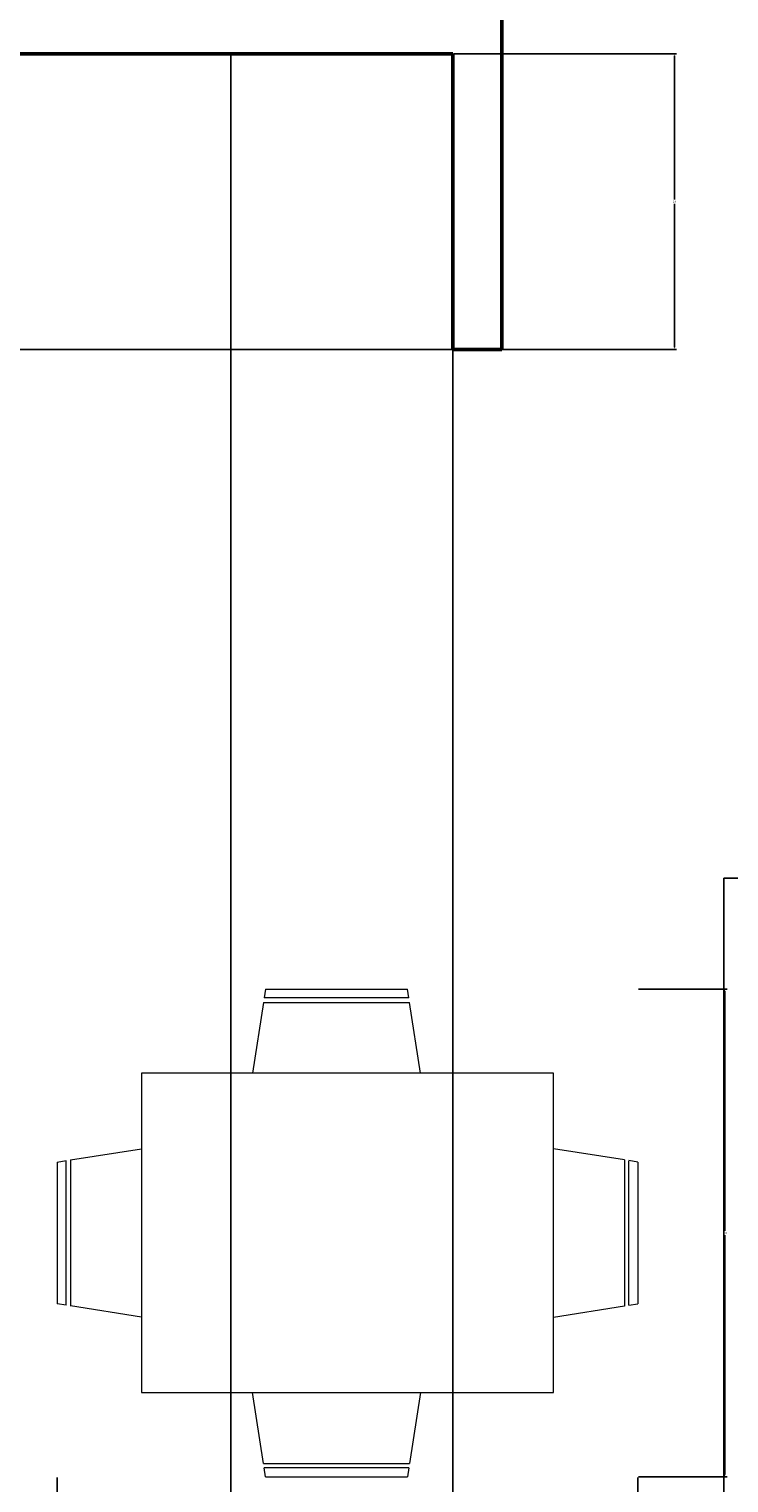
# Model space of a CAD drawing. Units: inches. Extents: x 2621 to 2849, y 2066 to 2463.
# Tile 11 of 28: x 2729 to 2786, y 2199 to 2317. Entities that reach past the tile are written whole.
import ezdxf

# ---------------------------------------------------------------- set-up
doc = ezdxf.new("R2010")
doc.units = ezdxf.units.IN
for name, color, linetype, lineweight in [('A-ANNO-DIMS', 2, 'Continuous', 18), ('A-FLOR-CASE', 9, 'Continuous', 25), ('A-FLOR-STRS', 7, 'Continuous', 25), ('A-FURN', 8, 'Continuous', 18), ('A-WALL', 7, 'Continuous', 50)]:
    doc.layers.add(name, color=color, linetype=linetype, lineweight=lineweight)
doc.styles.get("Standard").update_dxf_attribs({"font": 'arial.ttf'})
doc.dimstyles.get("Standard").update_dxf_attribs({"dimtxt": 0.18, "dimasz": 0.18, "dimexe": 0.18, "dimexo": 0.0625, "dimgap": 0.09, "dimtad": 0, "dimtih": 1, "dimtoh": 1, "dimdec": 4, "dimzin": 0, "dimdsep": 46, "dimtxsty": 'Standard', "dimcen": 0.09, "dimadec": 0, "dimazin": 0, "dimtfac": 1, "dimtdec": 4, "dimtofl": 0, "dimtmove": 0, "dimatfit": 3, "dimfxl": 1, "dimtolj": 1, "dimtzin": 0, "dimarcsym": 0})

# ---------------------------------------------------------------- blocks, each defined once
blk = doc.blocks.new('Dining Set - 36 x 72 in.')
for p, q in [((-22, 27.5), (-22.16, 26.5)), ((-5.84, 26.5), (-22.15, 26.5)), ((-22, 27.5), (-6, 27.5)), ((-5.84, 26.5), (-6, 27.5)), ((-22.23, 26), (-23.48, 18)), ((-22.23, 26), (-5.76, 26)), ((-4.52, 18), (-5.77, 26)), ((-36, 18), (-36, -18)), ((-0.18, 18), (-36, 18)), ((-2.03, 18), (-2.03, 18)), ((10.48, 18), (-0.18, 18)), ((10.48, -18), (10.48, 18)), ((-44, 8.23), (-36, 9.48)), ((-44, 8.23), (-44, -8.24)), ((18.49, 8.23), (10.48, 9.48)), ((18.48, 8.23), (18.48, -8.24)), ((-45.5, 8), (-44.5, 8.16)), ((-45.5, 8), (-45.5, -8)), ((-44.5, -8.16), (-44.5, 8.15)), ((18.98, -8.16), (18.98, 8.15)), ((19.98, 8), (18.99, 8.16)), ((19.98, 8), (19.98, -8)), ((-44.5, -8.16), (-45.5, -8)), ((18.98, -8.16), (19.98, -8)), ((-36, -9.48), (-44, -8.23)), ((10.48, -9.48), (18.48, -8.23)), ((-36, -18), (-0.18, -18)), ((-22.23, -26), (-23.48, -18)), ((-4.52, -18), (-5.77, -26)), ((-0.18, -18), (10.48, -18)), ((-22.23, -26), (-5.76, -26)), ((-22, -27.5), (-22.16, -26.5)), ((-5.84, -26.5), (-22.15, -26.5)), ((-22, -27.5), (-6, -27.5)), ((-5.84, -26.5), (-6, -27.5))]:
    blk.add_line(p, q)
blk = doc.blocks.new('*D25')
at = {"layer": 'A-ANNO-DIMS', "color": 0, "lineweight": -2, "transparency": 16777216}
for p, q in [((2731.76, 2199.81), (2731.76, 2192.62)), ((2778.9, 2199.81), (2778.9, 2192.62)), ((2731.94, 2192.8), (2754.36, 2192.8)), ((2778.72, 2192.8), (2756.3, 2192.8))]:
    blk.add_line(p, q, dxfattribs=at)
at = {"layer": 'A-ANNO-DIMS', "color": 0, "transparency": 16777216}
for points in [[(2731.94, 2192.83), (2731.94, 2192.77), (2731.76, 2192.8)], [(2778.72, 2192.83), (2778.72, 2192.77), (2778.9, 2192.8)]]:
    blk.add_solid(points, dxfattribs=at)
at = {"layer": 'Defpoints', "color": 0, "transparency": 16777216}
for p in [(2731.76, 2199.87), (2778.9, 2199.87), (2778.9, 2192.8)]:
    blk.add_point(p, dxfattribs=at)
at = {"layer": 'A-ANNO-DIMS', "color": 0, "transparency": 16777216, "insert": (2755.33, 2192.8), "char_height": 0.18, "attachment_point": 5}
blk.add_mtext('\\A1;DINING SET 47', dxfattribs=at)
blk = doc.blocks.new('*D26')
at = {"layer": 'A-ANNO-DIMS', "color": 0, "lineweight": -2, "transparency": 16777216}
for p, q in [((2778.96, 2239.46), (2786.15, 2239.46)), ((2785.97, 2239.28), (2785.97, 2219.84)), ((2785.97, 2200.05), (2785.97, 2219.48)), ((2778.96, 2199.87), (2786.15, 2199.87))]:
    blk.add_line(p, q, dxfattribs=at)
at = {"layer": 'A-ANNO-DIMS', "color": 0, "transparency": 16777216}
for points in [[(2785.94, 2239.28), (2786, 2239.28), (2785.97, 2239.46)], [(2785.94, 2200.05), (2786, 2200.05), (2785.97, 2199.87)]]:
    blk.add_solid(points, dxfattribs=at)
at = {"layer": 'Defpoints', "color": 0, "transparency": 16777216}
for p in [(2778.9, 2239.46), (2785.97, 2239.46), (2778.9, 2199.87)]:
    blk.add_point(p, dxfattribs=at)
at = {"layer": 'A-ANNO-DIMS', "color": 0, "transparency": 16777216, "insert": (2785.97, 2219.66), "char_height": 0.18, "attachment_point": 5}
blk.add_mtext('\\A1;40', dxfattribs=at)
blk = doc.blocks.new('*D69')
at = {"layer": 'A-ANNO-DIMS', "color": 0, "lineweight": -2, "transparency": 16777216}
for p, q in [((2763.93, 2315.37), (2782.05, 2315.37)), ((2781.87, 2315.19), (2781.87, 2303.55)), ((2781.87, 2291.55), (2781.87, 2303.19)), ((2763.93, 2291.37), (2782.05, 2291.37))]:
    blk.add_line(p, q, dxfattribs=at)
at = {"layer": 'A-ANNO-DIMS', "color": 0, "transparency": 16777216}
for points in [[(2781.84, 2315.19), (2781.9, 2315.19), (2781.87, 2315.37)], [(2781.84, 2291.55), (2781.9, 2291.55), (2781.87, 2291.37)]]:
    blk.add_solid(points, dxfattribs=at)
at = {"layer": 'Defpoints', "color": 0, "transparency": 16777216}
for p in [(2763.87, 2315.37), (2763.87, 2291.37), (2781.87, 2291.37)]:
    blk.add_point(p, dxfattribs=at)
at = {"layer": 'A-ANNO-DIMS', "color": 0, "transparency": 16777216, "insert": (2781.87, 2303.37), "char_height": 0.18, "attachment_point": 5}
blk.add_mtext('\\A1;24', dxfattribs=at)
blk = doc.blocks.new('*D70')
at = {"layer": 'A-ANNO-DIMS', "color": 0, "lineweight": -2, "transparency": 16777216}
for p, q in [((2745.86, 2291.31), (2745.86, 2066.19)), ((2763.87, 2291.31), (2763.87, 2066.19)), ((2746.04, 2066.37), (2754.41, 2066.37)), ((2763.69, 2066.37), (2755.32, 2066.37))]:
    blk.add_line(p, q, dxfattribs=at)
at = {"layer": 'A-ANNO-DIMS', "color": 0, "transparency": 16777216}
for points in [[(2746.04, 2066.4), (2746.04, 2066.34), (2745.86, 2066.37)], [(2763.69, 2066.4), (2763.69, 2066.34), (2763.87, 2066.37)]]:
    blk.add_solid(points, dxfattribs=at)
at = {"layer": 'Defpoints', "color": 0, "transparency": 16777216}
for p in [(2745.86, 2291.37), (2763.87, 2291.37), (2763.87, 2066.37)]:
    blk.add_point(p, dxfattribs=at)
at = {"layer": 'A-ANNO-DIMS', "color": 0, "transparency": 16777216, "insert": (2754.86, 2066.37), "char_height": 0.18, "attachment_point": 5}
blk.add_mtext('\\A1;18.014', dxfattribs=at)

msp = doc.modelspace()

# ---------------------------------------------------------------- linework, layer by layer
at = {"layer": 'A-FLOR-CASE'}
for p, q in [((2745.8562, 2291.3746), (2745.8562, 2315.3746)), ((2671.8701, 2291.3746), (2763.8701, 2291.3746))]:
    msp.add_line(p, q, dxfattribs=at)
at = {"layer": 'A-FLOR-STRS'}
for p, q in [((2821.8701, 2248.4598), (2785.8701, 2248.4598)), ((2785.8701, 2248.4598), (2785.8701, 2158.4598))]:
    msp.add_line(p, q, dxfattribs=at)
at = {"layer": 'A-WALL'}
for p, q in [((2767.8701, 2315.3746), (2767.8701, 2325.3746)), ((2647.8701, 2315.3746), (2763.8701, 2315.3746)), ((2763.8701, 2291.3746), (2763.8701, 2315.3746)), ((2767.8701, 2315.3746), (2767.8701, 2291.3746)), ((2767.8701, 2291.3746), (2763.8701, 2291.3746))]:
    msp.add_line(p, q, dxfattribs=at)

# ---------------------------------------------------------------- block references
at = {"layer": 'A-FURN', "xscale": 0.7197536828811776, "yscale": 0.7197536828811776, "zscale": 0.7197536828811776}
msp.add_blockref('Dining Set - 36 x 72 in.', (2764.5116, 2219.663), dxfattribs=at)

# ---------------------------------------------------------------- dimensions: what is measured, and where the dimension line sits
at = {"layer": 'A-ANNO-DIMS'}
for base, p1, p2, angle, picture, middle in [((2781.8736, 2291.3746), (2763.8701, 2315.3746), (2763.8701, 2291.3746), 270, '*D69', (2781.8736, 2303.3746)), ((2785.9656, 2239.4562), (2778.8957, 2199.8698), (2778.8957, 2239.4562), 90, '*D26', (2785.9656, 2219.663))]:
    dim = msp.add_linear_dim(base=base, p1=p1, p2=p2, angle=angle, dimstyle='Standard', override={"dimdec": 0, "dimlfac": 1, "dimrnd": 0, "dimzin": 0, "dimdsep": 46, "dimlunit": 2}, dxfattribs=at)
    dim.commit()
    dim.dimension.update_dxf_attribs({"geometry": picture, "text_midpoint": middle})
dim = msp.add_linear_dim(base=(2763.8701, 2066.3711), p1=(2745.8562, 2291.3746), p2=(2763.8701, 2291.3746), dimstyle='Standard', override={"dimdec": 3, "dimlfac": 1, "dimrnd": 0, "dimzin": 0, "dimdsep": 46, "dimlunit": 2}, dxfattribs=at)
dim.commit()
dim.dimension.update_dxf_attribs({"geometry": '*D70', "text_midpoint": (2754.8631, 2066.3711)})
dim = msp.add_linear_dim(base=(2778.8957, 2192.7999), p1=(2731.7628, 2199.8698), p2=(2778.8957, 2199.8698), text='DINING SET <>', dimstyle='Standard', override={"dimdec": 0, "dimlfac": 1, "dimrnd": 0, "dimzin": 0, "dimdsep": 46, "dimlunit": 2}, dxfattribs=at)
dim.commit()
dim.dimension.update_dxf_attribs({"geometry": '*D25', "text_midpoint": (2755.3293, 2192.7999)})

doc.saveas('drawing.dxf')
